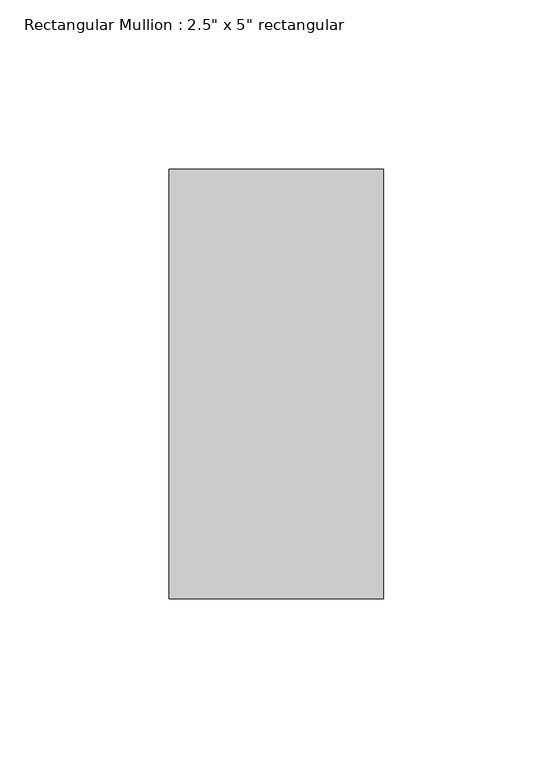
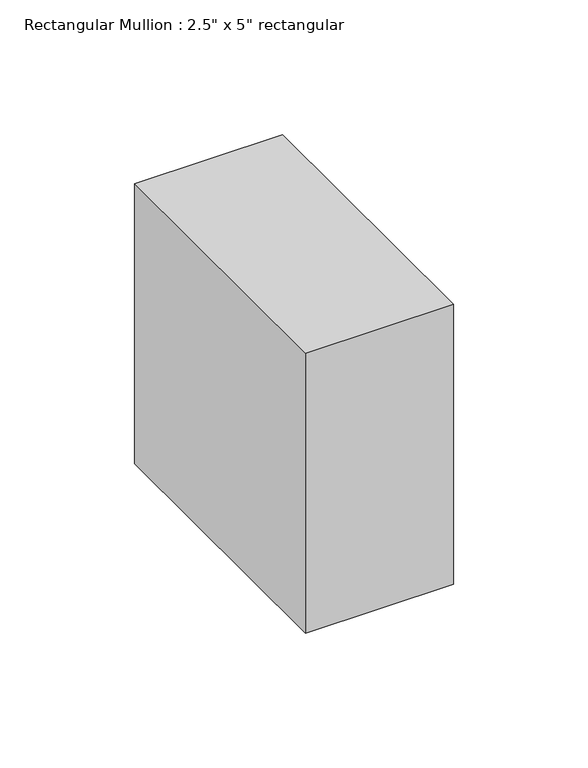
"""IFC4 building model written with IfcOpenShell, lengths in millimetres: member geometry."""

from ifc_helpers import new_model, si_unit, frame, origin, place, context, project, spatial, polyline, outline, extrude, source, transform, mapped, element, save


def member_a8e3eee7(model_context):
    return source(origin(), model_context, "Body", "SweptSolid", [
        extrude(outline(polyline([(0.0, 63.5), (0.0, -63.5), (-63.5, -63.5), (-63.5, 63.5), (0.0, 63.5)])), frame((0.0, 0.0, -127.0), z_axis=(0.0, 0.0, 1.0), x_axis=(1.0, 0.0, 0.0)), (0.0, 0.0, 1.0), 127.0),
    ])


if __name__ == "__main__":
    model = new_model("IFC4")
    model_context = context("Model", 3, world=origin())
    ifc_project = project(units=[si_unit("LENGTHUNIT", "METRE", prefix="MILLI")], contexts=[model_context])
    site = spatial("IfcSite", under=ifc_project)
    building = spatial("IfcBuilding", under=site)
    placement = place(None, origin())
    member_shape = member_a8e3eee7(model_context)
    element("IfcMember", 1, ObjectType="Rectangular Mullion : 2.5\" x 5\" rectangular", at=placement, inside=building, context=model_context, shape_type="MappedRepresentation", body=[
        mapped(member_shape, transform((0.0, 0.0, 0.0), x_axis=(1.0, 0.0, 0.0), y_axis=(0.0, 1.0, 0.0), z_axis=(0.0, 0.0, 1.0))),
    ])
    save(model, "model.ifc")

# Revit data of these elements
# Type "Rectangular Mullion : 2.5\" x 5\" rectangular"
#   built-in parameter 1007304 = 0.416667 (stored number, unit not read)
#   built-in parameter 1007301 = 0.104167 (stored number, unit not read)
#   built-in parameter 1007300 = 0.104167 (stored number, unit not read)
# Element 1 (IfcMember, "Rectangular Mullion : 2.5\" x 5\" rectangular")
#   Materials on its faces: "Aluminum"
# Materials
#   "Aluminum": class "Metal", colour RGB 247 247 247, transparency 0, Description = "Aluminum 6061", Cost = 0
